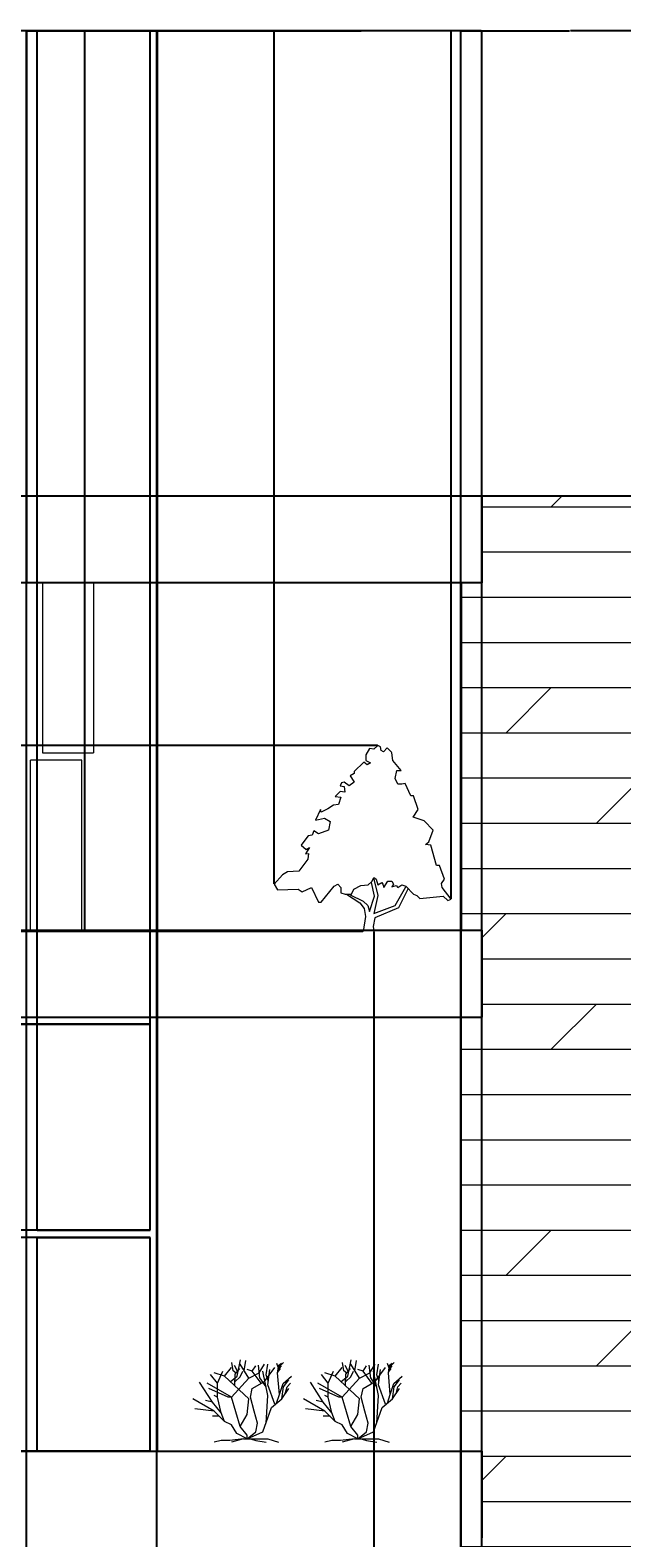
# Model space of a CAD drawing. Units: inches. Extents: x 250 to 1217, y -42 to 832.
# Tile 4 of 7: x 506 to 670, y 415 to 832. Entities that reach past the tile are written whole.
import ezdxf

# ---------------------------------------------------------------- set-up
doc = ezdxf.new("R2010")
doc.units = ezdxf.units.IN
doc.header["$MEASUREMENT"] = 0
for name, color, linetype, lineweight in [('A-ANNO-DIMS', 2, 'Continuous', 18), ('A-ELEV', 7, 'Continuous', 25), ('A-ELEV-PATT', 8, 'Continuous', 13), ('A-GLAZ', 4, 'Continuous', 18), ('L-PLNT', 3, 'Continuous', 13)]:
    doc.layers.add(name, color=color, linetype=linetype, lineweight=lineweight)
doc.styles.get("Standard").update_dxf_attribs({"font": 'arial.ttf'})
doc.dimstyles.get("Standard").update_dxf_attribs({"dimtxt": 0.18, "dimasz": 0.18, "dimexe": 0.18, "dimexo": 0.0625, "dimgap": 0.09, "dimtad": 0, "dimtih": 1, "dimtoh": 1, "dimdec": 4, "dimzin": 0, "dimdsep": 46, "dimtxsty": 'Standard', "dimcen": 0.09, "dimadec": 0, "dimazin": 0, "dimtfac": 1, "dimtdec": 4, "dimtofl": 0, "dimtmove": 0, "dimatfit": 3, "dimfxl": 1, "dimtolj": 1, "dimtzin": 0, "dimarcsym": 0})

# ---------------------------------------------------------------- blocks, each defined once
blk = doc.blocks.new('*U2')
for p, q in [((-12.471, 19.775), (-12.898, 22.044)), ((-11.28, 19.619), (-12.104, 21.184)), ((-11.433, 18.289), (-10.457, 22.749)), ((-8.16, 17.76), (-10.56, 21.6)), ((-9.48, 19.775), (-8.992, 22.592)), ((-7.2, 19.68), (-6.24, 21.12)), ((-5.086, 17.741), (-5.513, 21.34)), ((-5.28, 19.2), (-3.84, 21.6)), ((-3.377, 18.602), (-2.888, 21.575)), ((-0.508, 21.888), (-0.081, 20.558)), ((-0.203, 19.149), (0.102, 21.34)), ((-0.02, 20.01), (0.896, 21.105)), ((0.041, 20.714), (1.384, 22.044)), ((0.102, 21.34), (0.835, 21.888)), ((-16.8, 16.32), (-18.72, 18.72)), ((-14.88, 18.24), (-17.76, 19.2)), ((-16.8, 16.32), (-15.36, 19.68)), ((-14.88, 18.24), (-12.96, 20.64)), ((-8.16, 12), (-14.88, 18.24)), ((-13.325, 16.724), (-11.433, 18.289)), ((-12.96, 12.48), (-8.16, 17.76)), ((-11.677, 19.071), (-12.471, 19.775)), ((-12.043, 15.628), (-11.921, 18.836)), ((-11.982, 16.802), (-10.579, 18.054)), ((-11.921, 18.836), (-10.64, 20.401)), ((-10.579, 18.054), (-9.846, 19.697)), ((-7.2, 19.68), (-8.64, 20.16)), ((-8.16, 17.76), (-5.28, 19.2)), ((-4.8, 16.32), (-7.2, 19.68)), ((-7.2, 14.88), (-3.84, 16.8)), ((-3.377, 15.315), (-5.086, 17.819)), ((-2.88, 12.96), (-4.32, 19.68)), ((-3.84, 16.8), (-0.96, 20.64)), ((-2.766, 16.802), (-3.377, 18.602)), ((-2.88, 15.84), (-2.4, 20.16)), ((0.346, 13.203), (-0.203, 19.149)), ((-0.142, 19.384), (0.59, 20.401)), ((1.323, 16.254), (3.642, 18.289)), ((1.44, 15.36), (2.88, 17.28)), ((-18.24, 11.04), (-21.755, 16.655)), ((-12.96, 12.48), (-19.68, 16.32)), ((-13.92, 12.48), (-19.2, 14.88)), ((-16.8, 12.48), (-17.76, 12.96)), ((-16.8, 12.48), (-16.8, 16.32)), ((-7.68, 12.48), (-7.2, 14.88)), ((-3.36, 5.28), (-2.88, 12.96)), ((-0.96, 10.56), (-2.88, 15.84)), ((-0.48, 10.8), (0.346, 13.203)), ((0.346, 13.203), (1.323, 16.254)), ((0.96, 12), (1.44, 15.36)), ((0.96, 12), (2.88, 14.88)), ((1.92, 13.44), (2.4, 15.36)), ((2.4, 15.36), (3.36, 16.32)), ((-17.76, 8.64), (-23.663, 11.961)), ((-17.76, 8.64), (-23.128, 9.222)), ((-18.24, 11.04), (-20.16, 11.52)), ((-15.84, 8.16), (-18.24, 11.04)), ((-14.88, 5.76), (-17.76, 8.64)), ((-15.84, 8.16), (-16.8, 12.48)), ((-12.96, 12.48), (-13.92, 12.48)), ((-10.56, 4.32), (-12.96, 12.48)), ((-8.64, 7.68), (-8.16, 12)), ((-6.72, 8.64), (-7.68, 12.48)), ((-5.76, 5.28), (-6.72, 8.64)), ((-4.32, 2.88), (-1.92, 9.6)), ((-1.92, 9.6), (0.96, 12)), ((-16.32, 7.2), (-18.24, 7.2)), ((-14.88, 5.76), (-15.84, 8.16)), ((-12.96, 4.8), (-14.88, 5.76)), ((-11.52, 2.4), (-12.96, 4.8)), ((-10.56, 4.32), (-8.64, 7.68)), ((-8.64, 1.92), (-10.56, 4.32)), ((-6.24, 2.88), (-5.76, 5.28)), ((-15.84, 0.48), (-17.76, 0)), ((-13.44, 0.48), (-15.84, 0.48)), ((-9.6, 0.96), (-13.44, 0.48)), ((-9.6, 0.96), (-12.96, 0)), ((-8.64, 0.96), (-11.52, 2.4)), ((-9.6, 0.96), (-7.68, 0.96)), ((-8.64, 0.96), (-4.32, 2.88)), ((-8.64, 0.96), (-6.24, 2.88)), ((-8.64, 0.96), (-8.64, 1.92)), ((-8.64, 0.96), (-2.88, 0.96)), ((-7.68, 0.96), (-6.24, 0.48)), ((-6.24, 0.48), (-3.36, 0)), ((-2.88, 0.96), (0, 0))]:
    blk.add_line(p, q)
blk = doc.blocks.new('*U3')
for points in [[(22.0124, 137.721), (18.5475, 141.5624), (15.5282, 138.2446), (13.8028, 139.3505), (13.3714, 142.1153), (11.2148, 143.2214), (8.1954, 140.4564), (4.7447, 141.0094), (2.1567, 136.0326), (2.1567, 131.6088), (5.6074, 129.9499), (3.0193, 128.2909), (0.4313, 130.5029), (-6.9015, 123.3141), (-6.9015, 121.6552), (-9.9208, 119.9963), (-9.0581, 118.3373), (-6.9015, 115.0195), (-10.7835, 112.2546), (-14.6656, 115.0195), (-16.8222, 114.4665), (-17.6849, 112.2546), (-14.6656, 111.7016), (-14.2342, 107.2778), (-17.6065, 107.8307), (-21.5669, 103.9599), (-17.2536, 103.4069), (-18.9789, 97.8771), (-22.8609, 97.3241), (-27.1743, 94.5593), (-32.3504, 91.7944), (-32.7817, 94.0063), (-36.6638, 85.7116), (-29.7624, 87.3705), (-25.449, 84.6056), (-26.743, 77.9699), (-34.507, 75.205), (-37.9578, 77.4169), (-39.2518, 74.099), (-42.2711, 73.5461), (-44.8592, 70.2282), (-47.8786, 66.3574), (-43.9965, 63.0395), (-41.4085, 64.6985), (-44.3346, 59.8898), (-42.2089, 60.1377), (-42.5159, 55.7849), (-49.6039, 46.4502), (-58.2307, 45.8972), (-62.1127, 43.6853), (-68.5828, 36.4966), (-65.9947, 32.0727), (-50.0352, 32.6257), (-47.0159, 30.4138), (-39.6831, 33.7317), (-34.507, 22.6721), (-32.3504, 22.6721), (-22.4296, 34.8376), (-19.4102, 36.4966), (-17.2536, 33.7317), (-17.2536, 29.8608), (-13.8028, 28.7549), (-9.0581, 28.7549), (-7.3328, 32.6257), (-1.7254, 35.3906), (3.8821, 35.9436), (6.4701, 38.1555), (6.9014, 38.7085), (8.1954, 41.4734), (9.9208, 40.3674), (11.2148, 35.9436), (14.2341, 37.6025), (15.0968, 36.4966), (15.9595, 33.7317), (18.9789, 38.7085), (21.9982, 38.7085), (23.2922, 36.4966), (21.9982, 34.2847), (25.4489, 35.3906), (26.743, 33.7317), (29.7623, 35.9436), (32.7817, 34.8376), (38.8204, 28.7549), (41.4084, 27.6489), (43.5651, 25.437), (61.6813, 27.0959), (65.132, 23.7781), (67.7201, 24.884), (60.8186, 33.7317), (60.3873, 37.0495), (62.544, 40.3674), (58.662, 50.874), (56.5053, 50.874), (52.1919, 66.3574), (47.8785, 66.9103), (50.4665, 69.1222), (53.9172, 77.9699), (47.0158, 85.1586), (38.3891, 87.9235), (42.2711, 94.0063)], [(42.2711, 94.0063), (38.8204, 104.5129), (36.6637, 104.5129), (32.3503, 113.9135), (29.7623, 113.3605), (26.743, 113.3605), (24.5862, 117.7844), (25.8802, 123.8671), (29.331, 123.8671), (22.8609, 131.6088), (21.9982, 137.6916)], [(-9.9208, 28.2019), (0, 23.2251), (3.4507, 19.9072), (4.7447, 15.4834), (8.6267, 27.0959), (6.4701, 37.6025)], [(8.1954, 40.3674), (11.2148, 27.6489), (8.1954, 13.8245), (24.5862, 19.9072), (32.7817, 34.2847)], [(-12.9401, 28.7549), (-2.588, 22.1191), (0.8626, 17.6953), (1.7253, 11.6125), (0, 0)], [(34.5071, 33.1787), (27.1743, 18.2483), (9.0581, 10.5066), (7.7641, 3.8708), (8.1954, 0)]]:
    blk.add_lwpolyline(points)
blk = doc.blocks.new('WIN-PANEL-NARROW')
for p, q in [((0, 47), (0, 0)), ((14.16, 47), (14.16, 0)), ((0, 0), (14.16, 0))]:
    blk.add_line(p, q)
blk = doc.blocks.new('*D8')
at = {"layer": 'A-ANNO-DIMS', "color": 0, "lineweight": -2, "transparency": 16777216}
for p, q in [((352.34, 702.99), (352.34, 831.77)), ((352.52, 831.59), (491.1, 831.59)), ((630.6, 831.59), (492.03, 831.59)), ((630.78, 702.99), (630.78, 831.77))]:
    blk.add_line(p, q, dxfattribs=at)
at = {"layer": 'A-ANNO-DIMS', "color": 0, "transparency": 16777216}
for points in [[(352.52, 831.62), (352.52, 831.56), (352.34, 831.59)], [(630.6, 831.62), (630.6, 831.56), (630.78, 831.59)]]:
    blk.add_solid(points, dxfattribs=at)
at = {"layer": 'Defpoints', "color": 0, "transparency": 16777216}
for p in [(630.78, 831.59), (352.34, 702.93), (630.78, 702.93)]:
    blk.add_point(p, dxfattribs=at)
at = {"layer": 'A-ANNO-DIMS', "color": 0, "transparency": 16777216, "insert": (491.56, 831.59), "char_height": 0.18, "attachment_point": 5}
blk.add_mtext('\\A1;278.44', dxfattribs=at)
blk = doc.blocks.new('*D9')
at = {"layer": 'A-ANNO-DIMS', "color": 0, "lineweight": -2, "transparency": 16777216}
for p, q in [((630.78, 702.99), (630.78, 831.77)), ((630.96, 831.59), (654.6, 831.59)), ((679.01, 831.59), (655.36, 831.59)), ((679.19, 702.99), (679.19, 831.77))]:
    blk.add_line(p, q, dxfattribs=at)
at = {"layer": 'A-ANNO-DIMS', "color": 0, "transparency": 16777216}
for points in [[(630.96, 831.62), (630.96, 831.56), (630.78, 831.59)], [(679.01, 831.62), (679.01, 831.56), (679.19, 831.59)]]:
    blk.add_solid(points, dxfattribs=at)
at = {"layer": 'Defpoints', "color": 0, "transparency": 16777216}
for p in [(679.19, 831.59), (630.78, 702.93), (679.19, 702.93)]:
    blk.add_point(p, dxfattribs=at)
at = {"layer": 'A-ANNO-DIMS', "color": 0, "transparency": 16777216, "insert": (654.98, 831.59), "char_height": 0.18, "attachment_point": 5}
blk.add_mtext('\\A1;48.41', dxfattribs=at)
blk = doc.blocks.new('*D25')
at = {"layer": 'A-ANNO-DIMS', "color": 0, "lineweight": -2, "transparency": 16777216}
for p, q in [((504.98, 174.99), (504.98, 831.77)), ((505.16, 831.59), (522.76, 831.59)), ((540.8, 831.59), (523.2, 831.59)), ((540.98, 174.99), (540.98, 831.77))]:
    blk.add_line(p, q, dxfattribs=at)
at = {"layer": 'A-ANNO-DIMS', "color": 0, "transparency": 16777216}
for points in [[(505.16, 831.62), (505.16, 831.56), (504.98, 831.59)], [(540.8, 831.62), (540.8, 831.56), (540.98, 831.59)]]:
    blk.add_solid(points, dxfattribs=at)
at = {"layer": 'Defpoints', "color": 0, "transparency": 16777216}
for p in [(540.98, 831.59), (504.98, 174.93), (540.98, 174.93)]:
    blk.add_point(p, dxfattribs=at)
at = {"layer": 'A-ANNO-DIMS', "color": 0, "transparency": 16777216, "insert": (522.98, 831.59), "char_height": 0.18, "attachment_point": 5}
blk.add_mtext('\\A1;36', dxfattribs=at)
blk = doc.blocks.new('*D26')
at = {"layer": 'A-ANNO-DIMS', "color": 0, "lineweight": -2, "transparency": 16777216}
for p, q in [((540.98, 174.99), (540.98, 831.77)), ((541.16, 831.59), (582.76, 831.59)), ((624.8, 831.59), (583.2, 831.59)), ((624.98, 174.99), (624.98, 831.77))]:
    blk.add_line(p, q, dxfattribs=at)
at = {"layer": 'A-ANNO-DIMS', "color": 0, "transparency": 16777216}
for points in [[(541.16, 831.62), (541.16, 831.56), (540.98, 831.59)], [(624.8, 831.62), (624.8, 831.56), (624.98, 831.59)]]:
    blk.add_solid(points, dxfattribs=at)
at = {"layer": 'Defpoints', "color": 0, "transparency": 16777216}
for p in [(624.98, 831.59), (540.98, 174.93), (624.98, 174.93)]:
    blk.add_point(p, dxfattribs=at)
at = {"layer": 'A-ANNO-DIMS', "color": 0, "transparency": 16777216, "insert": (582.98, 831.59), "char_height": 0.18, "attachment_point": 5}
blk.add_mtext('\\A1;84', dxfattribs=at)
blk = doc.blocks.new('*D27')
at = {"layer": 'A-ANNO-DIMS', "color": 0, "lineweight": -2, "transparency": 16777216}
for p, q in [((624.98, 174.99), (624.98, 831.77)), ((625.16, 831.59), (655.07, 831.59)), ((685.76, 831.59), (655.86, 831.59)), ((685.94, 176.49), (685.94, 831.77))]:
    blk.add_line(p, q, dxfattribs=at)
at = {"layer": 'A-ANNO-DIMS', "color": 0, "transparency": 16777216}
for points in [[(625.16, 831.62), (625.16, 831.56), (624.98, 831.59)], [(685.76, 831.62), (685.76, 831.56), (685.94, 831.59)]]:
    blk.add_solid(points, dxfattribs=at)
at = {"layer": 'Defpoints', "color": 0, "transparency": 16777216}
for p in [(685.94, 831.59), (685.94, 176.43), (624.98, 174.93)]:
    blk.add_point(p, dxfattribs=at)
at = {"layer": 'A-ANNO-DIMS', "color": 0, "transparency": 16777216, "insert": (655.46, 831.59), "char_height": 0.18, "attachment_point": 5}
blk.add_mtext('\\A1;60.96', dxfattribs=at)
blk = doc.blocks.new('*D43')
at = {"layer": 'A-ANNO-DIMS', "color": 0, "lineweight": -2, "transparency": 16777216}
for p, q in [((505.06, 678.99), (505.06, 831.77)), ((505.24, 831.59), (512.61, 831.59)), ((520.89, 831.59), (513.52, 831.59)), ((521.07, 678.99), (521.07, 831.77))]:
    blk.add_line(p, q, dxfattribs=at)
at = {"layer": 'A-ANNO-DIMS', "color": 0, "transparency": 16777216}
for points in [[(505.24, 831.62), (505.24, 831.56), (505.06, 831.59)], [(520.89, 831.62), (520.89, 831.56), (521.07, 831.59)]]:
    blk.add_solid(points, dxfattribs=at)
at = {"layer": 'Defpoints', "color": 0, "transparency": 16777216}
for p in [(521.07, 831.59), (505.06, 678.93), (521.07, 678.93)]:
    blk.add_point(p, dxfattribs=at)
at = {"layer": 'A-ANNO-DIMS', "color": 0, "transparency": 16777216, "insert": (513.07, 831.59), "char_height": 0.18, "attachment_point": 5}
blk.add_mtext('\\A1;16.002', dxfattribs=at)
blk = doc.blocks.new('*D44')
at = {"layer": 'A-ANNO-DIMS', "color": 0, "lineweight": -2, "transparency": 16777216}
for p, q in [((521.07, 678.99), (521.07, 831.77)), ((521.25, 831.59), (572.79, 831.59)), ((624.88, 831.59), (573.35, 831.59)), ((625.06, 678.99), (625.06, 831.77))]:
    blk.add_line(p, q, dxfattribs=at)
at = {"layer": 'A-ANNO-DIMS', "color": 0, "transparency": 16777216}
for points in [[(521.25, 831.62), (521.25, 831.56), (521.07, 831.59)], [(624.88, 831.62), (624.88, 831.56), (625.06, 831.59)]]:
    blk.add_solid(points, dxfattribs=at)
at = {"layer": 'Defpoints', "color": 0, "transparency": 16777216}
for p in [(625.06, 831.59), (521.07, 678.93), (625.06, 678.93)]:
    blk.add_point(p, dxfattribs=at)
at = {"layer": 'A-ANNO-DIMS', "color": 0, "transparency": 16777216, "insert": (573.07, 831.59), "char_height": 0.18, "attachment_point": 5}
blk.add_mtext('\\A1;104', dxfattribs=at)
blk = doc.blocks.new('*D49')
at = {"layer": 'A-ANNO-DIMS', "color": 0, "lineweight": -2, "transparency": 16777216}
for p, q in [((348.98, 318.99), (348.98, 831.77)), ((349.16, 831.59), (489.48, 831.59)), ((630.6, 831.59), (490.28, 831.59)), ((630.78, 318.99), (630.78, 831.77))]:
    blk.add_line(p, q, dxfattribs=at)
at = {"layer": 'A-ANNO-DIMS', "color": 0, "transparency": 16777216}
for points in [[(349.16, 831.62), (349.16, 831.56), (348.98, 831.59)], [(630.6, 831.62), (630.6, 831.56), (630.78, 831.59)]]:
    blk.add_solid(points, dxfattribs=at)
at = {"layer": 'Defpoints', "color": 0, "transparency": 16777216}
for p in [(630.78, 831.59), (348.98, 318.93), (630.78, 318.93)]:
    blk.add_point(p, dxfattribs=at)
at = {"layer": 'A-ANNO-DIMS', "color": 0, "transparency": 16777216, "insert": (489.88, 831.59), "char_height": 0.18, "attachment_point": 5}
blk.add_mtext('\\A1;281.8', dxfattribs=at)
blk = doc.blocks.new('*D54')
at = {"layer": 'A-ANNO-DIMS', "color": 0, "lineweight": -2, "transparency": 16777216}
for p, q in [((408.52, 440.1), (408.52, 831.77)), ((408.7, 831.59), (474.4, 831.59)), ((541, 831.59), (475.31, 831.59)), ((541.18, 438.99), (541.18, 831.77))]:
    blk.add_line(p, q, dxfattribs=at)
at = {"layer": 'A-ANNO-DIMS', "color": 0, "transparency": 16777216}
for points in [[(408.7, 831.62), (408.7, 831.56), (408.52, 831.59)], [(541, 831.62), (541, 831.56), (541.18, 831.59)]]:
    blk.add_solid(points, dxfattribs=at)
at = {"layer": 'Defpoints', "color": 0, "transparency": 16777216}
for p in [(541.18, 831.59), (408.52, 440.03), (541.18, 438.93)]:
    blk.add_point(p, dxfattribs=at)
at = {"layer": 'A-ANNO-DIMS', "color": 0, "transparency": 16777216, "insert": (474.85, 831.59), "char_height": 0.18, "attachment_point": 5}
blk.add_mtext('\\A1;132.66', dxfattribs=at)
blk = doc.blocks.new('*D82')
at = {"layer": 'A-ANNO-DIMS', "color": 0, "lineweight": -2, "transparency": 16777216}
for p, q in [((507.88, 556.99), (507.88, 831.77)), ((508.06, 831.59), (523.14, 831.59)), ((539, 831.59), (523.92, 831.59)), ((539.18, 556.99), (539.18, 831.77))]:
    blk.add_line(p, q, dxfattribs=at)
at = {"layer": 'A-ANNO-DIMS', "color": 0, "transparency": 16777216}
for points in [[(508.06, 831.62), (508.06, 831.56), (507.88, 831.59)], [(539, 831.62), (539, 831.56), (539.18, 831.59)]]:
    blk.add_solid(points, dxfattribs=at)
at = {"layer": 'Defpoints', "color": 0, "transparency": 16777216}
for p in [(539.18, 831.59), (507.88, 556.93), (539.18, 556.93)]:
    blk.add_point(p, dxfattribs=at)
at = {"layer": 'A-ANNO-DIMS', "color": 0, "transparency": 16777216, "insert": (523.53, 831.59), "char_height": 0.18, "attachment_point": 5}
blk.add_mtext('\\A1;31.30', dxfattribs=at)
blk = doc.blocks.new('*D83')
at = {"layer": 'A-ANNO-DIMS', "color": 0, "lineweight": -2, "transparency": 16777216}
for p, q in [((539.12, 497.99), (250.36, 497.99)), ((250.54, 497.81), (250.54, 468.64)), ((250.54, 439.11), (250.54, 468.28)), ((539.12, 438.93), (250.36, 438.93))]:
    blk.add_line(p, q, dxfattribs=at)
at = {"layer": 'A-ANNO-DIMS', "color": 0, "transparency": 16777216}
for points in [[(250.51, 497.81), (250.57, 497.81), (250.54, 497.99)], [(250.51, 439.11), (250.57, 439.11), (250.54, 438.93)]]:
    blk.add_solid(points, dxfattribs=at)
at = {"layer": 'Defpoints', "color": 0, "transparency": 16777216}
for p in [(250.54, 497.99), (539.18, 497.99), (539.18, 438.93)]:
    blk.add_point(p, dxfattribs=at)
at = {"layer": 'A-ANNO-DIMS', "color": 0, "transparency": 16777216, "insert": (250.54, 468.46), "char_height": 0.18, "attachment_point": 5}
blk.add_mtext('\\A1;59.06', dxfattribs=at)
blk = doc.blocks.new('*D84')
at = {"layer": 'A-ANNO-DIMS', "color": 0, "lineweight": -2, "transparency": 16777216}
for p, q in [((539.12, 499.99), (250.36, 499.99)), ((539.12, 497.99), (250.36, 497.99)), ((250.54, 499.81), (250.54, 499.17)), ((250.54, 498.17), (250.54, 498.81))]:
    blk.add_line(p, q, dxfattribs=at)
at = {"layer": 'A-ANNO-DIMS', "color": 0, "transparency": 16777216}
for points in [[(250.51, 499.81), (250.57, 499.81), (250.54, 499.99)], [(250.51, 498.17), (250.57, 498.17), (250.54, 497.99)]]:
    blk.add_solid(points, dxfattribs=at)
at = {"layer": 'Defpoints', "color": 0, "transparency": 16777216}
for p in [(250.54, 499.99), (539.18, 499.99), (539.18, 497.99)]:
    blk.add_point(p, dxfattribs=at)
at = {"layer": 'A-ANNO-DIMS', "color": 0, "transparency": 16777216, "insert": (250.54, 498.99), "char_height": 0.18, "attachment_point": 5}
blk.add_mtext('\\A1;2.00', dxfattribs=at)
blk = doc.blocks.new('*D85')
at = {"layer": 'A-ANNO-DIMS', "color": 0, "lineweight": -2, "transparency": 16777216}
for p, q in [((539.12, 556.93), (250.36, 556.93)), ((250.54, 556.75), (250.54, 528.64)), ((250.54, 500.17), (250.54, 528.28)), ((539.12, 499.99), (250.36, 499.99))]:
    blk.add_line(p, q, dxfattribs=at)
at = {"layer": 'A-ANNO-DIMS', "color": 0, "transparency": 16777216}
for points in [[(250.51, 556.75), (250.57, 556.75), (250.54, 556.93)], [(250.51, 500.17), (250.57, 500.17), (250.54, 499.99)]]:
    blk.add_solid(points, dxfattribs=at)
at = {"layer": 'Defpoints', "color": 0, "transparency": 16777216}
for p in [(250.54, 556.93), (539.18, 556.93), (539.18, 499.99)]:
    blk.add_point(p, dxfattribs=at)
at = {"layer": 'A-ANNO-DIMS', "color": 0, "transparency": 16777216, "insert": (250.54, 528.46), "char_height": 0.18, "attachment_point": 5}
blk.add_mtext('\\A1;56.94', dxfattribs=at)
blk = doc.blocks.new('*D93')
at = {"layer": 'A-ANNO-DIMS', "color": 0, "lineweight": -2, "transparency": 16777216}
for p, q in [((573.41, 595.74), (573.41, 831.77)), ((573.59, 831.59), (597.47, 831.59)), ((622.15, 831.59), (598.27, 831.59)), ((622.33, 591.58), (622.33, 831.77))]:
    blk.add_line(p, q, dxfattribs=at)
at = {"layer": 'A-ANNO-DIMS', "color": 0, "transparency": 16777216}
for points in [[(573.59, 831.62), (573.59, 831.56), (573.41, 831.59)], [(622.15, 831.62), (622.15, 831.56), (622.33, 831.59)]]:
    blk.add_solid(points, dxfattribs=at)
at = {"layer": 'Defpoints', "color": 0, "transparency": 16777216}
for p in [(622.33, 831.59), (573.41, 595.68), (622.33, 591.51)]:
    blk.add_point(p, dxfattribs=at)
at = {"layer": 'A-ANNO-DIMS', "color": 0, "transparency": 16777216, "insert": (597.87, 831.59), "char_height": 0.18, "attachment_point": 5}
blk.add_mtext('\\A1;48.92', dxfattribs=at)
blk = doc.blocks.new('*D94')
at = {"layer": 'A-ANNO-DIMS', "color": 0, "lineweight": -2, "transparency": 16777216}
for p, q in [((601.99, 633.99), (250.36, 633.99)), ((250.54, 633.81), (250.54, 608.47)), ((250.54, 582.76), (250.54, 608.1)), ((597.96, 582.58), (250.36, 582.58))]:
    blk.add_line(p, q, dxfattribs=at)
at = {"layer": 'A-ANNO-DIMS', "color": 0, "transparency": 16777216}
for points in [[(250.51, 633.81), (250.57, 633.81), (250.54, 633.99)], [(250.51, 582.76), (250.57, 582.76), (250.54, 582.58)]]:
    blk.add_solid(points, dxfattribs=at)
at = {"layer": 'Defpoints', "color": 0, "transparency": 16777216}
for p in [(250.54, 633.99), (602.05, 633.99), (598.03, 582.58)]:
    blk.add_point(p, dxfattribs=at)
at = {"layer": 'A-ANNO-DIMS', "color": 0, "transparency": 16777216, "insert": (250.54, 608.29), "char_height": 0.18, "attachment_point": 5}
blk.add_mtext('\\A1;51.41', dxfattribs=at)
blk = doc.blocks.new('*D95')
at = {"layer": 'A-ANNO-DIMS', "color": 0, "lineweight": -2, "transparency": 16777216}
for p, q in [((600.97, 582.52), (600.97, -41.6)), ((625.06, 582.86), (625.06, -41.6)), ((601.15, -41.42), (612.62, -41.42)), ((624.88, -41.42), (613.41, -41.42))]:
    blk.add_line(p, q, dxfattribs=at)
at = {"layer": 'A-ANNO-DIMS', "color": 0, "transparency": 16777216}
for points in [[(601.15, -41.39), (601.15, -41.45), (600.97, -41.42)], [(624.88, -41.39), (624.88, -41.45), (625.06, -41.42)]]:
    blk.add_solid(points, dxfattribs=at)
at = {"layer": 'Defpoints', "color": 0, "transparency": 16777216}
for p in [(600.97, 582.58), (625.06, 582.93), (625.06, -41.42)]:
    blk.add_point(p, dxfattribs=at)
at = {"layer": 'A-ANNO-DIMS', "color": 0, "transparency": 16777216, "insert": (613.02, -41.42), "char_height": 0.18, "attachment_point": 5}
blk.add_mtext('\\A1;24.10', dxfattribs=at)

msp = doc.modelspace()

# ---------------------------------------------------------------- hatches: boundary and pattern name
at = {"layer": 'A-ELEV-PATT'}
h = msp.add_hatch(dxfattribs=at)
h.set_pattern_fill('DOLMIT', color=256, scale=50)
h.paths.add_polyline_path([(684.9826, 558.9271), (679.1872, 558.9271), (679.1872, 582.9271), (685.0649, 582.9271), (685.0649, 678.9271), (679.1872, 678.9271), (679.1872, 702.9271), (630.7779, 702.9271), (630.7779, 678.9271), (625.0649, 678.9271), (625.0649, 582.9271), (630.7779, 582.9271), (630.7779, 558.9271), (624.9826, 558.9271), (624.9826, 438.9271), (630.7779, 438.9271), (630.7779, 414.9271), (624.9826, 414.9271), (624.9826, 318.9271), (630.7779, 318.9271), (630.7779, 294.9271), (624.9826, 294.9271), (624.9826, 198.9271), (630.7779, 198.9271), (630.7779, 174.9271), (624.9826, 174.9271), (624.9826, 78.9271), (684.9826, 78.9271), (684.9826, 174.9271), (679.1872, 174.9271), (679.1872, 198.9271), (683.6004, 198.9271), (684.9826, 198.9271), (684.9826, 294.9271), (679.1872, 294.9271), (679.1872, 318.9271), (684.9826, 318.9271), (684.9826, 414.9271), (679.1872, 414.9271), (679.1872, 438.9271), (684.9826, 438.9271)])

# ---------------------------------------------------------------- linework, layer by layer
at = {"layer": 'A-ELEV'}
for p, q in [((630.7779, 702.9271), (630.7779, 678.9271)), ((521.0669, 582.9271), (521.0669, 678.9271)), ((625.0649, 678.9271), (625.0649, 582.9271)), ((376.3429, 582.9271), (630.7779, 582.9271)), ((376.3429, 582.9271), (630.7779, 582.9271)), ((630.7779, 582.9271), (630.7779, 558.9271)), ((352.3429, 558.9271), (630.7779, 558.9271)), ((408.9826, 558.9271), (541.1795, 558.9271)), ((541.1795, 438.9271), (541.1795, 558.9271)), ((624.9826, 558.9271), (624.9826, 438.9271)), ((410.9826, 556.9271), (539.1795, 556.9271)), ((507.8802, 499.991), (507.8802, 556.9271)), ((539.1795, 499.991), (539.1795, 556.9271)), ((507.8802, 499.991), (539.1795, 499.991)), ((507.8802, 438.9271), (507.8802, 497.991)), ((507.8802, 497.991), (539.1795, 497.991)), ((539.1795, 438.9271), (539.1795, 497.991)), ((352.3429, 438.9271), (630.7779, 438.9271)), ((630.7779, 438.9271), (630.7779, 414.9271))]:
    msp.add_line(p, q, dxfattribs=at)
for points in [[(952.2329, 582.9271), (952.2329, 702.9271), (352.3429, 702.9271), (352.3429, 582.9271)], [(630.7779, 678.9271), (376.3429, 678.9271), (376.3429, 582.9271)]]:
    msp.add_lwpolyline(points, dxfattribs=at)

# ---------------------------------------------------------------- block references
at = {"layer": 'A-GLAZ'}
msp.add_blockref('WIN-PANEL-NARROW', (509.3428, 631.927), dxfattribs=at)
at = {"layer": 'A-GLAZ', "rotation": 180}
msp.add_blockref('WIN-PANEL-NARROW', (520.2282, 629.9271), dxfattribs=at)
at = {"layer": 'L-PLNT', "xscale": 0.3589292991008459, "yscale": 0.3589292991008459, "zscale": 0.3589292991008459}
msp.add_blockref('*U3', (598.0256, 582.5825), dxfattribs=at)
at = {"layer": 'L-PLNT'}
for p in [(574.5796, 441.3562), (605.1804, 441.3562)]:
    msp.add_blockref('*U2', p, dxfattribs=at)

# ---------------------------------------------------------------- dimensions: what is measured, and where the dimension line sits
at = {"layer": 'A-ANNO-DIMS'}
for base, p1, p2, override, picture, middle in [((630.7779, 831.5941), (348.9826, 318.9271), (630.7779, 318.9271), {"dimdec": 1, "dimlfac": 1, "dimrnd": 0, "dimzin": 0, "dimdsep": 46, "dimlunit": 2}, '*D49', (489.8803, 831.5941)), ((630.77793, 831.59407), (352.34291, 702.92707), (630.77793, 702.92707), {"dimdec": 2, "dimlfac": 1, "dimrnd": 0, "dimzin": 0, "dimdsep": 46, "dimlunit": 2}, '*D8', (491.56042, 831.59407)), ((541.1795, 831.5941), (408.5234, 440.0339), (541.1795, 438.9271), {"dimdec": 2, "dimlfac": 1, "dimrnd": 0, "dimzin": 0, "dimdsep": 46, "dimlunit": 2}, '*D54', (474.8515, 831.5941)), ((540.9826, 831.5941), (504.9826, 174.9271), (540.9826, 174.9271), {"dimdec": 0, "dimlfac": 1, "dimrnd": 0, "dimzin": 0, "dimdsep": 46, "dimlunit": 2}, '*D25', (522.9826, 831.5941)), ((521.0669, 831.5941), (505.0649, 678.9271), (521.0669, 678.9271), {"dimdec": 3, "dimlfac": 1, "dimrnd": 0, "dimzin": 0, "dimdsep": 46, "dimlunit": 2}, '*D43', (513.0659, 831.5941)), ((539.1795, 831.5941), (507.8802, 556.9271), (539.1795, 556.9271), {"dimdec": 2, "dimlfac": 1, "dimrnd": 0, "dimzin": 0, "dimdsep": 46, "dimlunit": 2}, '*D82', (523.5298, 831.5941)), ((625.0649, 831.5941), (521.0669, 678.9271), (625.0649, 678.9271), {"dimdec": 0, "dimlfac": 1, "dimrnd": 0, "dimzin": 0, "dimdsep": 46, "dimlunit": 2}, '*D44', (573.0659, 831.5941)), ((624.9826, 831.5941), (540.9826, 174.9271), (624.9826, 174.9271), {"dimdec": 0, "dimlfac": 1, "dimrnd": 0, "dimzin": 0, "dimdsep": 46, "dimlunit": 2}, '*D26', (582.9826, 831.5941)), ((622.3324, 831.5941), (573.4093, 595.6822), (622.3324, 591.5141), {"dimdec": 2, "dimlfac": 1, "dimrnd": 0, "dimzin": 0, "dimdsep": 46, "dimlunit": 2}, '*D93', (597.8708, 831.5941)), ((685.944, 831.5941), (624.9826, 174.9271), (685.944, 176.4321), {"dimdec": 2, "dimlfac": 1, "dimrnd": 0, "dimzin": 0, "dimdsep": 46, "dimlunit": 2}, '*D27', (655.4633, 831.5941)), ((679.1872, 831.5941), (630.7779, 702.9271), (679.1872, 702.9271), {"dimdec": 2, "dimlfac": 1, "dimrnd": 0, "dimzin": 0, "dimdsep": 46, "dimlunit": 2}, '*D9', (654.9826, 831.5941)), ((625.0649, -41.4199), (600.9672, 582.5825), (625.0649, 582.9271), {"dimdec": 2, "dimlfac": 1, "dimrnd": 0, "dimzin": 0, "dimdsep": 46, "dimlunit": 2}, '*D95', (613.0161, -41.4199))]:
    dim = msp.add_linear_dim(base=base, p1=p1, p2=p2, dimstyle='Standard', override=override, dxfattribs=at)
    dim.commit()
    dim.dimension.update_dxf_attribs({"geometry": picture, "text_midpoint": middle})
for base, p1, p2, picture, middle in [((250.5369, 633.9889), (598.0256, 582.5825), (602.051, 633.9889), '*D94', (250.5369, 608.2857)), ((250.5369, 556.9271), (539.1795, 499.991), (539.1795, 556.9271), '*D85', (250.5369, 528.459)), ((250.5369, 497.991), (539.1795, 438.9271), (539.1795, 497.991), '*D83', (250.5369, 468.459)), ((250.5369, 499.991), (539.1795, 497.991), (539.1795, 499.991), '*D84', (250.5369, 498.991))]:
    dim = msp.add_linear_dim(base=base, p1=p1, p2=p2, angle=90, dimstyle='Standard', override={"dimdec": 2, "dimlfac": 1, "dimrnd": 0, "dimzin": 0, "dimdsep": 46, "dimlunit": 2}, dxfattribs=at)
    dim.commit()
    dim.dimension.update_dxf_attribs({"geometry": picture, "text_midpoint": middle})

doc.saveas('drawing.dxf')
